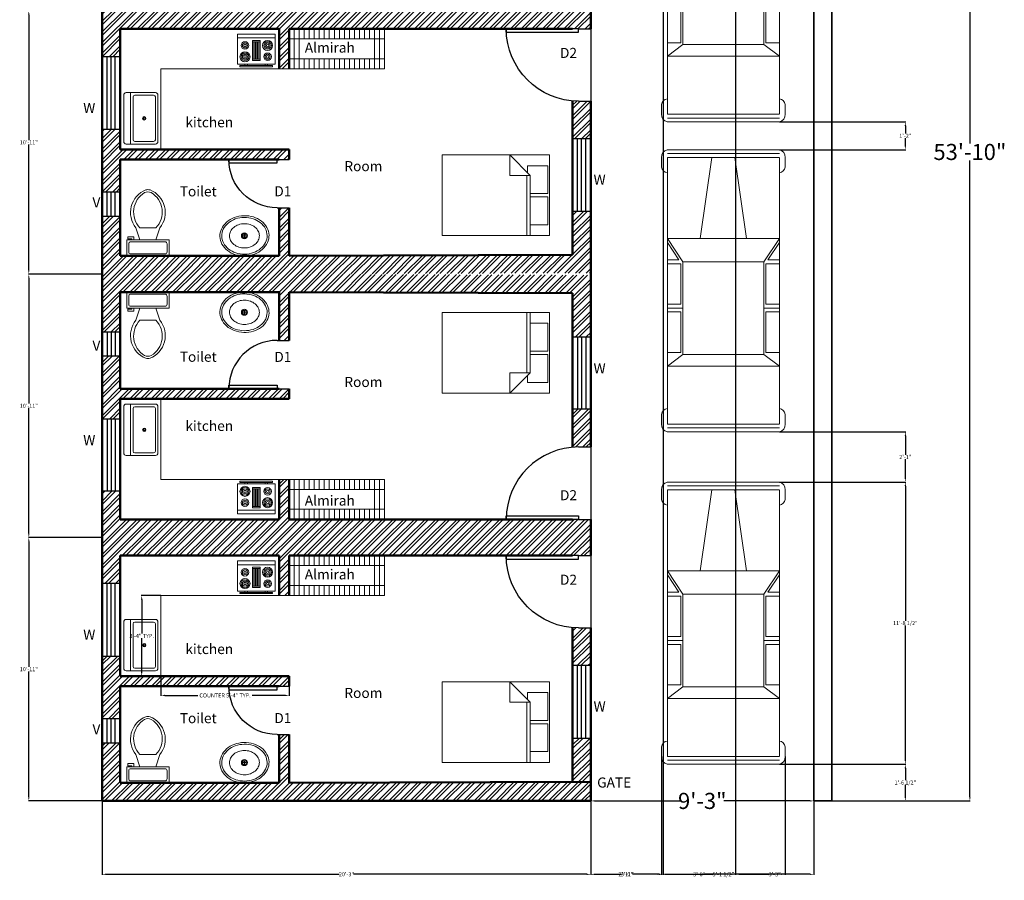
# Model space of a CAD drawing. Units: inches. Extents: x -83 to 408, y 158 to 919.
# Tile 1 of 5: x -82 to 408, y 158 to 586. Entities that reach past the tile are written whole.
import ezdxf

# ---------------------------------------------------------------- set-up
doc = ezdxf.new("R2010")
doc.units = ezdxf.units.IN
doc.header["$MEASUREMENT"] = 0
for name, color, linetype, lineweight in [('A-ANNO-DIMS', 2, 'Continuous', 18), ('A-ANNO-TEXT', 7, 'Continuous', 18), ('A-AREA-IDEN', 7, 'Continuous', 18), ('A-DOOR', 3, 'Continuous', 25), ('A-EQPM', 8, 'Continuous', 18), ('A-FLOR-CASE', 30, 'Continuous', 18), ('A-FLOR-FIXT', 9, 'Continuous', 18), ('A-FURN', 8, 'Continuous', 18), ('A-GLAZ', 4, 'Continuous', 25), ('A-WALL', 7, 'Continuous', 50), ('A-WALL-PATT', 252, 'Continuous', 13), ('C-PKNG-VEHI', 8, 'Continuous', 18), ('L-WALL', 7, 'Continuous', 35)]:
    doc.layers.add(name, color=color, linetype=linetype, lineweight=lineweight)
doc.styles.get("Standard").update_dxf_attribs({"font": 'arial.ttf'})
doc.dimstyles.get("Standard").update_dxf_attribs({"dimtxt": 2, "dimasz": 2, "dimexe": 0.18, "dimexo": 0.0625, "dimgap": 0.09, "dimtad": 0, "dimtih": 1, "dimtoh": 1, "dimdec": 0, "dimzin": 0, "dimdsep": 46, "dimlunit": 3, "dimtxsty": 'Standard', "dimcen": 0.09, "dimadec": 0, "dimazin": 0, "dimtfac": 1, "dimtdec": 0, "dimtofl": 0, "dimtmove": 0, "dimatfit": 3, "dimfxl": 1, "dimtolj": 1, "dimtzin": 0, "dimarcsym": 0})
pattern_1 = [(45, (0, -122.02), (-2.65165, 2.65165), []), (45, (1.7678, -122.02), (-2.65165, 2.65165), [])]

# ---------------------------------------------------------------- blocks, each defined once
blk = doc.blocks.new('Sink - Oval top')
for p, q in [((-1, 0), (1, 0)), ((0, 1), (0, -1))]:
    blk.add_line(p, q)
for points in [[(-12.23, 0.39, 0.117634), (-11.46, -3.36, 0.104469), (-8.88, -6.8, 0.090016), (-5.08, -9.07, 0.08192), (-0.32, -10.02, 0.08192), (4.49, -9.38, 0.090016), (8.42, -7.36, 0.104469), (11.22, -4.09, 0.117634), (12.23, -0.39, 0.117634), (11.46, 3.36, 0.104469), (8.88, 6.8, 0.090016), (5.08, 9.07, 0.08192), (0.32, 10.02, 0.08192), (-4.49, 9.38, 0.090016), (-8.42, 7.36, 0.104469), (-11.22, 4.09, 0.117634)], [(-11.29, 0.16, 0.118622), (-10.52, -3.25, 0.104678), (-8.07, -6.36, 0.089562), (-4.54, -8.37, 0.081185), (-0.13, -9.15, 0.081185), (4.3, -8.49, 0.089562), (7.89, -6.58, 0.104678), (10.42, -3.55, 0.118622), (11.29, -0.16, 0.118622), (10.52, 3.25, 0.104678), (8.07, 6.36, 0.089562), (4.54, 8.37, 0.081185), (0.13, 9.15, 0.081185), (-4.3, 8.49, 0.089562), (-7.89, 6.58, 0.104678), (-10.42, 3.55, 0.118622)], [(-7.42, 0.08, 0.118283), (-6.91, -2.17, 0.104607), (-5.29, -4.21, 0.089718), (-2.97, -5.53, 0.081436), (-0.07, -6.04, 0.081436), (2.84, -5.59, 0.089718), (5.2, -4.33, 0.104607), (6.86, -2.32, 0.118283), (7.42, -0.08, 0.118283), (6.91, 2.17, 0.104607), (5.29, 4.21, 0.089718), (2.97, 5.53, 0.081436), (0.07, 6.04, 0.081436), (-2.84, 5.59, 0.089718), (-5.2, 4.33, 0.104607), (-6.86, 2.32, 0.118283)]]:
    blk.add_lwpolyline(points, format="xyb", close=True)
for radius in [1.5, 1]:
    blk.add_circle((0, 0), radius)
blk = doc.blocks.new('Toilet - top')
for p, q in [((9.5, -6), (9.5, -2)), ((-10, -8.5), (-8, -8.5)), ((-10, -9.5), (-10, -8.5)), ((-7, -9.5), (-10, -9.5)), ((-8, -8.5), (-8, -8)), ((-7, -8), (-7, -9.5)), ((-4, -8), (-6, -14)), ((4, -8), (6, -14)), ((4, -14), (-4, -14))]:
    blk.add_line(p, q)
blk.add_lwpolyline([(10.5, -8), (10.5, 0), (-10.5, 0), (-10.5, -8)], close=True)
for points in [[(-9.5, -2), (-9.5, -6)], [(8.5, -1), (-8.5, -1)], [(-8.5, -7), (8.5, -7)]]:
    blk.add_lwpolyline(points)
for centre, radius, start, end in [((-8.62, -1.88), 0.884, 81.8699, 188.1301), ((8.62, -1.88), 0.884, 351.8699, 98.1301), ((-8.62, -6.12), 0.884, 171.8699, 278.1301), ((8.62, -6.12), 0.884, 261.8699, 8.1301), ((3.52, -21.58), 12.17, 141.4691, 247.9714), ((4.2, -21.82), 11.33, 136.3677, 238.9468), ((-3.52, -21.58), 12.17, 292.0284, 38.5307), ((-4.2, -21.82), 11.33, 301.053, 43.6321), ((0, -27.88), 4, 245.7318, 294.2682), ((0, -29), 4, 254.8605, 285.1395)]:
    blk.add_arc(centre, radius, start, end)
blk = doc.blocks.new('Bed - Queen')
for p, q in [((0, -80.00003), (0, 0)), ((0, 0), (59.99999, 0)), ((59.99999, 0), (59.99999, -80.00003)), ((7.99999, -1.2), (28.79998, -1.2)), ((7.99999, -14.4), (7.99999, -1.2)), ((28.79998, -1.2), (28.79998, -14.4)), ((31.19999, -1.2), (51.99999, -1.2)), ((31.19999, -14.4), (31.19999, -1.2)), ((51.99999, -1.2), (51.99999, -16.4)), ((0, -14.4), (44.8, -14.4)), ((59.99999, -29.6), (44.8, -14.4)), ((44.8, -14.4), (44.8, -29.6)), ((44.8, -16.8), (0, -16.8)), ((51.99999, -16.4), (46.79936, -16.4)), ((44.8, -29.6), (59.99999, -29.6)), ((59.99999, -80.00003), (0, -80.00003))]:
    blk.add_line(p, q)
blk = doc.blocks.new('Sink-single - 30 in top')
blk.add_line((-15, -3.999996), (15, -3.999996))
for points in [[(-13.5, 0), (13.5, 0)], [(-15, -18.499996), (-15, -1.5)], [(-12.5, -5.499996), (12.5, -5.499996)], [(15, -1.5), (15, -18.499996)], [(-13.5, -17.499996), (-13.5, -6.499996)], [(13.5, -6.499996), (13.5, -17.499996)], [(13.5, -19.999996), (-13.5, -19.999996)], [(12.5, -18.499996), (-12.5, -18.499996)]]:
    blk.add_lwpolyline(points)
for radius in [1, 0.5]:
    blk.add_circle((0, -11.999996), radius)
for centre, radius, start, end in [((-13.5, -1.5), 1.5, 90, 180), ((-12.5, -6.499996), 1, 90, 180), ((12.5, -6.499996), 1, 0, 90), ((13.5, -1.5), 1.5, 0, 90), ((-13.5, -18.499996), 1.5, 180, 270), ((-12.5, -17.499996), 1, 180, 270), ((12.5, -17.499996), 1, 270, 0), ((13.5, -18.499996), 1.5, 270, 0)]:
    blk.add_arc(centre, radius, start, end)
blk = doc.blocks.new('Range-Oven - 30 in top')
for p, q in [((0, -3), (30, -3)), ((12, -6), (18, -6)), ((13, -20), (13, -6)), ((14, -6), (14, -20)), ((15, -20), (15, -6)), ((16, -6), (16, -20)), ((17, -20), (17, -6)), ((18, -20), (12, -20)), ((6, -24), (6, -25)), ((8, -25), (8, -24)), ((22, -25), (22, -24)), ((24, -24), (24, -25))]:
    blk.add_line(p, q)
for points in [[(0, -24), (0, 0), (30, 0), (30, -24)], [(12, -21), (12, -5), (18, -5), (18, -21)], [(2, -26), (2, -25), (28, -25), (28, -26)]]:
    blk.add_lwpolyline(points, close=True)
for centre, radius in [((6, -9), 4), ((6, -9), 3), ((6, -9), 2), ((24, -9), 3), ((24, -9), 2), ((6, -18), 3), ((6, -9), 1), ((24, -18), 4), ((24, -18), 3), ((24, -9), 1), ((6, -18), 2), ((6, -18), 1), ((24, -18), 2), ((24, -18), 1)]:
    blk.add_circle(centre, radius)
blk = doc.blocks.new('*U12')
for p, q in [((0, 0), (0, -6)), ((24, 0), (24, -6))]:
    blk.add_line(p, q)
blk.add_lwpolyline([(0, 0), (0, 24), (1.75, 24), (1.75, 0)], close=True)
blk.add_arc((0, 0), 24, 0, 90)
blk = doc.blocks.new('*U13')
for p, q in [((0, 0), (0, -6)), ((36, 0), (36, -6))]:
    blk.add_line(p, q)
blk.add_lwpolyline([(0, 0), (0, 36), (1.75, 36), (1.75, 0)], close=True)
blk.add_arc((0, 0), 36, 0, 90)
blk = doc.blocks.new('*U15')
for p, q in [((5.44, 42.31), (12.12, 42.31)), ((189.69, 42.31), (183.01, 42.31)), ((0.1, -0.41), (0.1, 38.35)), ((2.77, -0.41), (2.77, 38.31)), ((5.44, -0.41), (5.44, 38.24)), ((5.45, 38.31), (16.12, 38.31)), ((16.12, 38.31), (180.34, 38.31)), ((61.52, -0.41), (61.52, 38.31)), ((61.52, 38.31), (77.54, 27.62)), ((64.19, 38.31), (76.2, 30.29)), ((76.2, 30.29), (76.2, 38.31)), ((78.87, 38.31), (78.87, 28.96)), ((106.91, 28.96), (106.91, 38.31)), ((109.58, 27.62), (109.58, 38.31)), ((112.25, 38.31), (112.25, 28.96)), ((140.29, 28.96), (140.29, 38.31)), ((141.62, 27.62), (149.64, 38.31)), ((149.64, -0.41), (149.64, 38.31)), ((189.69, 38.31), (179.01, 38.31)), ((189.69, -0.41), (189.69, 38.24)), ((192.36, -0.41), (192.36, 38.31)), ((195.03, -0.41), (195.03, 38.35)), ((77.54, 27.62), (141.62, 27.62)), ((77.54, -0.41), (77.54, 27.62)), ((78.87, 28.96), (106.91, 28.96)), ((112.25, 28.96), (140.29, 28.96)), ((141.62, -0.41), (141.62, 27.62)), ((5.44, 7.6), (61.52, 15.61)), ((0.1, -0.42), (0.1, -39.18)), ((2.77, -0.41), (2.77, -39.13)), ((5.44, -0.42), (5.44, -39.07)), ((61.52, -0.41), (61.52, -39.13)), ((77.54, -0.41), (77.54, -28.45)), ((141.62, -0.41), (141.62, -28.45)), ((149.64, -0.41), (149.64, -39.13)), ((189.69, -0.42), (189.69, -39.07)), ((192.36, -0.41), (192.36, -39.13)), ((195.03, -0.42), (195.03, -39.18)), ((5.44, -8.42), (61.52, -16.43)), ((61.52, -39.13), (77.54, -28.45)), ((64.19, -39.13), (76.2, -31.12)), ((76.2, -31.12), (76.2, -39.13)), ((77.54, -28.45), (141.62, -28.45)), ((78.87, -39.13), (78.87, -29.79)), ((78.87, -29.79), (106.91, -29.79)), ((106.91, -29.79), (106.91, -39.13)), ((109.58, -28.45), (109.58, -39.13)), ((112.25, -29.79), (140.29, -29.79)), ((112.25, -39.13), (112.25, -29.79)), ((140.29, -29.79), (140.29, -39.13)), ((141.62, -28.45), (149.64, -39.13)), ((5.45, -39.13), (16.12, -39.13)), ((16.12, -39.13), (180.34, -39.13)), ((189.69, -39.13), (179.01, -39.13)), ((5.44, -43.14), (12.12, -43.14)), ((189.69, -43.14), (183.01, -43.14))]:
    blk.add_line(p, q)
for centre, radius, start, end in [((5.06, 37.26), 5.06, 85.64554, 168.0943), ((11.45, 37.64), 4.72, 8.13011, 81.86996), ((183.68, 37.64), 4.72, 98.13004, 171.8699), ((190.07, 37.26), 5.06, 11.90574, 94.35446), ((5.06, -38.09), 5.06, 191.9057, 274.3545), ((11.45, -38.46), 4.72, 278.13, 351.8699), ((183.68, -38.46), 4.72, 188.1301, 261.87), ((190.07, -38.09), 5.06, 265.6455, 348.0943)]:
    blk.add_arc(centre, radius, start, end)
blk = doc.blocks.new('*D16')
at = {"layer": 'A-ANNO-DIMS', "color": 0, "lineweight": -2, "transparency": 16777216}
for p, q in [((202.19, 197.1), (202.19, 196.97)), ((204.19, 197.15), (246.97, 197.15)), ((311.19, 197.15), (268.41, 197.15)), ((313.19, 197.21), (313.19, 197.33))]:
    blk.add_line(p, q, dxfattribs=at)
at = {"layer": 'A-ANNO-DIMS', "color": 0, "transparency": 16777216}
for points in [[(204.19, 197.48), (204.19, 196.82), (202.19, 197.15)], [(311.19, 197.48), (311.19, 196.82), (313.19, 197.15)]]:
    blk.add_solid(points, dxfattribs=at)
at = {"layer": 'Defpoints', "color": 0, "transparency": 16777216}
for p in [(202.19, 197.16), (313.19, 197.15), (313.19, 197.15)]:
    blk.add_point(p, dxfattribs=at)
at = {"layer": 'A-ANNO-DIMS', "color": 0, "transparency": 16777216, "insert": (257.69, 197.15), "char_height": 2, "attachment_point": 5}
blk.add_mtext('\\A1;{\\H4x;9\'-3"}', dxfattribs=at)
blk = doc.blocks.new('*D17')
at = {"layer": 'A-ANNO-DIMS', "color": 0, "lineweight": -2, "transparency": 16777216}
for p, q in [((322.25, 842.67), (390.98, 842.67)), ((390.8, 840.67), (390.8, 524.09)), ((390.8, 199.15), (390.8, 515.73)), ((322.25, 197.15), (390.98, 197.15))]:
    blk.add_line(p, q, dxfattribs=at)
at = {"layer": 'A-ANNO-DIMS', "color": 0, "transparency": 16777216}
for points in [[(390.47, 840.67), (391.14, 840.67), (390.8, 842.67)], [(390.47, 199.15), (391.14, 199.15), (390.8, 197.15)]]:
    blk.add_solid(points, dxfattribs=at)
at = {"layer": 'Defpoints', "color": 0, "transparency": 16777216}
for p in [(322.19, 842.67), (322.19, 197.15), (390.8, 197.15)]:
    blk.add_point(p, dxfattribs=at)
at = {"layer": 'A-ANNO-DIMS', "color": 0, "transparency": 16777216, "insert": (390.8, 519.91), "char_height": 2, "attachment_point": 5}
blk.add_mtext('\\A1;{\\H4x;53\'-10"}', dxfattribs=at)
blk = doc.blocks.new('ALMIRAH-47IN')
for p, q in [((0, 19.88), (47.48, 19.88)), ((0, 19.88), (0, 0)), ((2.48, 19.88), (2.48, 0)), ((4.98, 19.88), (4.98, 0)), ((7.48, 19.88), (7.48, 14.88)), ((9.98, 19.88), (9.98, 14.88)), ((9.98, 19.88), (9.98, 14.88)), ((9.98, 19.88), (9.98, 14.88)), ((12.48, 19.88), (12.48, 14.88)), ((14.98, 19.88), (14.98, 14.88)), ((14.98, 19.88), (14.98, 14.88)), ((17.48, 19.88), (17.48, 14.88)), ((19.98, 19.88), (19.98, 14.88)), ((22.48, 19.88), (22.48, 14.88)), ((22.48, 19.88), (22.48, 14.88)), ((24.98, 19.88), (24.98, 14.88)), ((24.98, 19.88), (24.98, 14.88)), ((27.48, 19.88), (27.48, 14.88)), ((29.98, 19.88), (29.98, 14.88)), ((29.98, 19.88), (29.98, 14.88)), ((29.98, 19.88), (29.98, 14.88)), ((32.48, 19.88), (32.48, 14.88)), ((34.98, 19.88), (34.98, 14.88)), ((37.48, 19.88), (37.48, 14.88)), ((39.98, 19.88), (39.98, 14.88)), ((42.48, 19.88), (42.48, 0)), ((44.98, 19.88), (44.98, 0)), ((47.48, 19.88), (47.48, 0)), ((0, 14.88), (47.48, 14.88)), ((0, 5), (47.48, 5)), ((7.48, 5), (7.48, 0)), ((9.98, 5), (9.98, 0)), ((9.98, 5), (9.98, 0)), ((9.98, 5), (9.98, 0)), ((12.48, 5), (12.48, 0)), ((14.98, 5), (14.98, 0)), ((14.98, 5), (14.98, 0)), ((17.48, 5), (17.48, 0)), ((19.98, 5), (19.98, 0)), ((22.48, 5), (22.48, 0)), ((22.48, 5), (22.48, 0)), ((24.98, 5), (24.98, 0)), ((24.98, 5), (24.98, 0)), ((27.48, 5), (27.48, 0)), ((29.98, 5), (29.98, 0)), ((29.98, 5), (29.98, 0)), ((29.98, 5), (29.98, 0)), ((32.48, 5), (32.48, 0)), ((34.98, 5), (34.98, 0)), ((37.48, 5), (37.48, 0)), ((39.98, 5), (39.98, 0))]:
    blk.add_line(p, q)
blk = doc.blocks.new('WINDOW-36IN')
for p, q in [((2.5, 36), (2.5, 0)), ((4.5, 36), (4.5, 0)), ((6.5, 36), (6.5, 0))]:
    blk.add_line(p, q)
blk.add_lwpolyline([(0, 36), (9, 36), (9, 0), (0, 0)], close=True)
blk = doc.blocks.new('VENT-12IN')
for p, q in [((2.5, 12), (2.5, 0)), ((4.5, 12), (4.5, 0)), ((6.5, 12), (6.5, 0))]:
    blk.add_line(p, q)
blk.add_lwpolyline([(0, 12), (9, 12), (9, 0), (0, 0)], close=True)
blk = doc.blocks.new('COUNTER-L-STUDIO')
for p, q in [((0, 40.12), (0, 40.12)), ((0, 40.12), (0, 0)), ((0, 0), (63.78, 0))]:
    blk.add_line(p, q)
blk = doc.blocks.new('*D39')
at = {"layer": 'A-ANNO-DIMS', "color": 0, "lineweight": -2, "transparency": 16777216}
for p, q in [((-11.59, 259.12), (-11.59, 249.43)), ((52.19, 259.12), (52.19, 249.43)), ((-9.59, 249.61), (6.83, 249.61)), ((50.19, 249.61), (33.77, 249.61))]:
    blk.add_line(p, q, dxfattribs=at)
at = {"layer": 'A-ANNO-DIMS', "color": 0, "transparency": 16777216}
for points in [[(-9.59, 249.95), (-9.59, 249.28), (-11.59, 249.61)], [(50.19, 249.95), (50.19, 249.28), (52.19, 249.61)]]:
    blk.add_solid(points, dxfattribs=at)
at = {"layer": 'Defpoints', "color": 0, "transparency": 16777216}
for p in [(-11.59, 259.18), (52.19, 259.18), (52.19, 249.61)]:
    blk.add_point(p, dxfattribs=at)
at = {"layer": 'A-ANNO-DIMS', "color": 0, "transparency": 16777216, "insert": (20.3, 249.61), "char_height": 2, "attachment_point": 5}
blk.add_mtext('\\A1;COUNTER 5\'-4" TYP.', dxfattribs=at)
blk = doc.blocks.new('*D40')
at = {"layer": 'A-ANNO-DIMS', "color": 0, "lineweight": -2, "transparency": 16777216}
for p, q in [((-11.66, 299.3), (-21.34, 299.3)), ((-21.16, 297.3), (-21.16, 280.35)), ((-21.16, 261.18), (-21.16, 278.13)), ((-11.66, 259.18), (-21.34, 259.18))]:
    blk.add_line(p, q, dxfattribs=at)
at = {"layer": 'A-ANNO-DIMS', "color": 0, "transparency": 16777216}
for points in [[(-21.49, 297.3), (-20.83, 297.3), (-21.16, 299.3)], [(-21.49, 261.18), (-20.83, 261.18), (-21.16, 259.18)]]:
    blk.add_solid(points, dxfattribs=at)
at = {"layer": 'Defpoints', "color": 0, "transparency": 16777216}
for p in [(-11.59, 299.3), (-21.16, 259.18), (-11.59, 259.18)]:
    blk.add_point(p, dxfattribs=at)
at = {"layer": 'A-ANNO-DIMS', "color": 0, "transparency": 16777216, "insert": (-21.16, 279.24), "char_height": 2, "attachment_point": 5}
blk.add_mtext('\\A1;3\'-4" TYP.', dxfattribs=at)
blk = doc.blocks.new('*D41')
at = {"layer": 'A-ANNO-DIMS', "color": 0, "lineweight": -2, "transparency": 16777216}
for p, q in [((-40.81, 197.12), (-40.81, 160.47)), ((202.19, 197.1), (202.19, 160.47)), ((-38.81, 160.65), (77.15, 160.65)), ((200.19, 160.65), (84.23, 160.65))]:
    blk.add_line(p, q, dxfattribs=at)
at = {"layer": 'A-ANNO-DIMS', "color": 0, "transparency": 16777216}
for points in [[(-38.81, 160.98), (-38.81, 160.32), (-40.81, 160.65)], [(200.19, 160.98), (200.19, 160.32), (202.19, 160.65)]]:
    blk.add_solid(points, dxfattribs=at)
at = {"layer": 'Defpoints', "color": 0, "transparency": 16777216}
for p in [(-40.81, 197.18), (202.19, 197.16), (202.19, 160.65)]:
    blk.add_point(p, dxfattribs=at)
at = {"layer": 'A-ANNO-DIMS', "color": 0, "transparency": 16777216, "insert": (80.69, 160.65), "char_height": 2, "attachment_point": 5}
blk.add_mtext('\\A1;20\'-3"', dxfattribs=at)
blk = doc.blocks.new('*D44')
at = {"layer": 'A-ANNO-DIMS', "color": 0, "lineweight": -2, "transparency": 16777216}
for p, q in [((-40.87, 590.18), (-77.49, 590.18)), ((-77.31, 588.18), (-77.31, 525.79)), ((-77.31, 461.18), (-77.31, 523.57)), ((-40.87, 459.18), (-77.49, 459.18))]:
    blk.add_line(p, q, dxfattribs=at)
at = {"layer": 'A-ANNO-DIMS', "color": 0, "transparency": 16777216}
for points in [[(-77.64, 588.18), (-76.98, 588.18), (-77.31, 590.18)], [(-77.64, 461.18), (-76.98, 461.18), (-77.31, 459.18)]]:
    blk.add_solid(points, dxfattribs=at)
at = {"layer": 'Defpoints', "color": 0, "transparency": 16777216}
for p in [(-40.81, 590.18), (-77.31, 459.18), (-40.81, 459.18)]:
    blk.add_point(p, dxfattribs=at)
at = {"layer": 'A-ANNO-DIMS', "color": 0, "transparency": 16777216, "insert": (-77.31, 524.68), "char_height": 2, "attachment_point": 5}
blk.add_mtext('\\A1;10\'-11"', dxfattribs=at)
blk = doc.blocks.new('*D45')
at = {"layer": 'A-ANNO-DIMS', "color": 0, "lineweight": -2, "transparency": 16777216}
for p, q in [((-40.87, 459.18), (-77.49, 459.18)), ((-77.31, 457.18), (-77.31, 394.79)), ((-77.31, 330.18), (-77.31, 392.57)), ((-40.87, 328.18), (-77.49, 328.18))]:
    blk.add_line(p, q, dxfattribs=at)
at = {"layer": 'A-ANNO-DIMS', "color": 0, "transparency": 16777216}
for points in [[(-77.64, 457.18), (-76.98, 457.18), (-77.31, 459.18)], [(-77.64, 330.18), (-76.98, 330.18), (-77.31, 328.18)]]:
    blk.add_solid(points, dxfattribs=at)
at = {"layer": 'Defpoints', "color": 0, "transparency": 16777216}
for p in [(-40.81, 459.18), (-77.31, 328.18), (-40.81, 328.18)]:
    blk.add_point(p, dxfattribs=at)
at = {"layer": 'A-ANNO-DIMS', "color": 0, "transparency": 16777216, "insert": (-77.31, 393.68), "char_height": 2, "attachment_point": 5}
blk.add_mtext('\\A1;10\'-11"', dxfattribs=at)
blk = doc.blocks.new('*D46')
at = {"layer": 'A-ANNO-DIMS', "color": 0, "lineweight": -2, "transparency": 16777216}
for p, q in [((-40.87, 328.18), (-77.49, 328.18)), ((-77.31, 326.18), (-77.31, 263.79)), ((-77.31, 199.18), (-77.31, 261.57)), ((-40.87, 197.18), (-77.49, 197.18))]:
    blk.add_line(p, q, dxfattribs=at)
at = {"layer": 'A-ANNO-DIMS', "color": 0, "transparency": 16777216}
for points in [[(-77.64, 326.18), (-76.98, 326.18), (-77.31, 328.18)], [(-77.64, 199.18), (-76.98, 199.18), (-77.31, 197.18)]]:
    blk.add_solid(points, dxfattribs=at)
at = {"layer": 'Defpoints', "color": 0, "transparency": 16777216}
for p in [(-40.81, 328.18), (-77.31, 197.18), (-40.81, 197.18)]:
    blk.add_point(p, dxfattribs=at)
at = {"layer": 'A-ANNO-DIMS', "color": 0, "transparency": 16777216, "insert": (-77.31, 262.68), "char_height": 2, "attachment_point": 5}
blk.add_mtext('\\A1;10\'-11"', dxfattribs=at)
blk = doc.blocks.new('*D57')
at = {"layer": 'A-ANNO-DIMS', "color": 0, "lineweight": -2, "transparency": 16777216}
for p, q in [((274.19, 685.53), (274.19, 160.47)), ((313.19, 685.53), (313.19, 160.47)), ((276.19, 160.65), (290.94, 160.65)), ((311.19, 160.65), (296.44, 160.65))]:
    blk.add_line(p, q, dxfattribs=at)
at = {"layer": 'A-ANNO-DIMS', "color": 0, "transparency": 16777216}
for points in [[(276.19, 160.98), (276.19, 160.32), (274.19, 160.65)], [(311.19, 160.98), (311.19, 160.32), (313.19, 160.65)]]:
    blk.add_solid(points, dxfattribs=at)
at = {"layer": 'Defpoints', "color": 0, "transparency": 16777216}
for p in [(274.19, 685.59), (313.19, 685.59), (313.19, 160.65)]:
    blk.add_point(p, dxfattribs=at)
at = {"layer": 'A-ANNO-DIMS', "color": 0, "transparency": 16777216, "insert": (293.69, 160.65), "char_height": 2, "attachment_point": 5}
blk.add_mtext('\\A1;3\'-3"', dxfattribs=at)
blk = doc.blocks.new('*D59')
at = {"layer": 'A-ANNO-DIMS', "color": 0, "lineweight": -2, "transparency": 16777216}
for p, q in [((202.19, 769.53), (202.19, 160.47)), ((238.19, 769.53), (238.19, 160.47)), ((204.19, 160.65), (217.44, 160.65)), ((236.19, 160.65), (222.94, 160.65))]:
    blk.add_line(p, q, dxfattribs=at)
at = {"layer": 'A-ANNO-DIMS', "color": 0, "transparency": 16777216}
for points in [[(204.19, 160.98), (204.19, 160.32), (202.19, 160.65)], [(236.19, 160.98), (236.19, 160.32), (238.19, 160.65)]]:
    blk.add_solid(points, dxfattribs=at)
at = {"layer": 'Defpoints', "color": 0, "transparency": 16777216}
for p in [(202.19, 769.59), (238.19, 769.59), (238.19, 160.65)]:
    blk.add_point(p, dxfattribs=at)
at = {"layer": 'A-ANNO-DIMS', "color": 0, "transparency": 16777216, "insert": (220.19, 160.65), "char_height": 2, "attachment_point": 5}
blk.add_mtext('\\A1;3\'-0"', dxfattribs=at)
blk = doc.blocks.new('*D60')
at = {"layer": 'A-ANNO-DIMS', "color": 0, "lineweight": -2, "transparency": 16777216}
for p, q in [((238.19, 805.53), (238.19, 160.47)), ((274.19, 805.53), (274.19, 160.47)), ((240.19, 160.65), (253.44, 160.65)), ((272.19, 160.65), (258.94, 160.65))]:
    blk.add_line(p, q, dxfattribs=at)
at = {"layer": 'A-ANNO-DIMS', "color": 0, "transparency": 16777216}
for points in [[(240.19, 160.98), (240.19, 160.32), (238.19, 160.65)], [(272.19, 160.98), (272.19, 160.32), (274.19, 160.65)]]:
    blk.add_solid(points, dxfattribs=at)
at = {"layer": 'Defpoints', "color": 0, "transparency": 16777216}
for p in [(238.19, 805.59), (274.19, 805.59), (274.19, 160.65)]:
    blk.add_point(p, dxfattribs=at)
at = {"layer": 'A-ANNO-DIMS', "color": 0, "transparency": 16777216, "insert": (256.19, 160.65), "char_height": 2, "attachment_point": 5}
blk.add_mtext('\\A1;3\'-0"', dxfattribs=at)
blk = doc.blocks.new('*D64')
at = {"layer": 'A-ANNO-DIMS', "color": 0, "lineweight": -2, "transparency": 16777216}
for p, q in [((237.43, 219.2), (237.43, 160.47)), ((202.19, 197.1), (202.19, 160.47)), ((204.19, 160.65), (216.27, 160.65)), ((235.43, 160.65), (223.35, 160.65))]:
    blk.add_line(p, q, dxfattribs=at)
at = {"layer": 'A-ANNO-DIMS', "color": 0, "transparency": 16777216}
for points in [[(204.19, 160.98), (204.19, 160.32), (202.19, 160.65)], [(235.43, 160.98), (235.43, 160.32), (237.43, 160.65)]]:
    blk.add_solid(points, dxfattribs=at)
at = {"layer": 'Defpoints', "color": 0, "transparency": 16777216}
for p in [(237.43, 219.26), (202.19, 197.16), (237.43, 160.65)]:
    blk.add_point(p, dxfattribs=at)
at = {"layer": 'A-ANNO-DIMS', "color": 0, "transparency": 16777216, "insert": (219.81, 160.65), "char_height": 2, "attachment_point": 5}
blk.add_mtext('\\A1;2\'-11"', dxfattribs=at)
blk = doc.blocks.new('*D65')
at = {"layer": 'A-ANNO-DIMS', "color": 0, "lineweight": -2, "transparency": 16777216}
for p, q in [((237.43, 219.2), (237.43, 160.47)), ((298.94, 219.2), (298.94, 160.47)), ((239.43, 160.65), (263.11, 160.65)), ((296.94, 160.65), (273.26, 160.65))]:
    blk.add_line(p, q, dxfattribs=at)
at = {"layer": 'A-ANNO-DIMS', "color": 0, "transparency": 16777216}
for points in [[(239.43, 160.98), (239.43, 160.32), (237.43, 160.65)], [(296.94, 160.98), (296.94, 160.32), (298.94, 160.65)]]:
    blk.add_solid(points, dxfattribs=at)
at = {"layer": 'Defpoints', "color": 0, "transparency": 16777216}
for p in [(237.43, 219.26), (298.94, 219.26), (298.94, 160.65)]:
    blk.add_point(p, dxfattribs=at)
at = {"layer": 'A-ANNO-DIMS', "color": 0, "transparency": 16777216, "insert": (268.18, 160.65), "char_height": 2, "attachment_point": 5}
blk.add_mtext('\\A1;5\'-1 1/2"', dxfattribs=at)
blk = doc.blocks.new('*D66')
at = {"layer": 'A-ANNO-DIMS', "color": 0, "lineweight": -2, "transparency": 16777216}
for p, q in [((296.12, 215.42), (358.87, 215.42)), ((358.69, 213.42), (358.69, 207.41)), ((358.69, 199.15), (358.69, 205.16)), ((313.25, 197.15), (358.87, 197.15))]:
    blk.add_line(p, q, dxfattribs=at)
at = {"layer": 'A-ANNO-DIMS', "color": 0, "transparency": 16777216}
for points in [[(358.36, 213.42), (359.02, 213.42), (358.69, 215.42)], [(358.36, 199.15), (359.02, 199.15), (358.69, 197.15)]]:
    blk.add_solid(points, dxfattribs=at)
at = {"layer": 'Defpoints', "color": 0, "transparency": 16777216}
for p in [(296.06, 215.42), (313.19, 197.15), (358.69, 197.15)]:
    blk.add_point(p, dxfattribs=at)
at = {"layer": 'A-ANNO-DIMS', "color": 0, "transparency": 16777216, "insert": (358.69, 206.28), "char_height": 2, "attachment_point": 5}
blk.add_mtext('\\A1;1\'-6 1/2"', dxfattribs=at)
blk = doc.blocks.new('*D67')
at = {"layer": 'A-ANNO-DIMS', "color": 0, "lineweight": -2, "transparency": 16777216}
for p, q in [((296.12, 355.73), (358.87, 355.73)), ((358.69, 353.73), (358.69, 286.7)), ((358.69, 217.42), (358.69, 284.45)), ((296.12, 215.42), (358.87, 215.42))]:
    blk.add_line(p, q, dxfattribs=at)
at = {"layer": 'A-ANNO-DIMS', "color": 0, "transparency": 16777216}
for points in [[(358.36, 353.73), (359.02, 353.73), (358.69, 355.73)], [(358.36, 217.42), (359.02, 217.42), (358.69, 215.42)]]:
    blk.add_solid(points, dxfattribs=at)
at = {"layer": 'Defpoints', "color": 0, "transparency": 16777216}
for p in [(296.06, 355.73), (358.69, 355.73), (296.06, 215.42)]:
    blk.add_point(p, dxfattribs=at)
at = {"layer": 'A-ANNO-DIMS', "color": 0, "transparency": 16777216, "insert": (358.69, 285.58), "char_height": 2, "attachment_point": 5}
blk.add_mtext('\\A1;11\'-8 1/2"', dxfattribs=at)
blk = doc.blocks.new('*D68')
at = {"layer": 'A-ANNO-DIMS', "color": 0, "lineweight": -2, "transparency": 16777216}
for p, q in [((296.12, 380.73), (358.87, 380.73)), ((358.69, 378.73), (358.69, 369.32)), ((358.69, 357.73), (358.69, 367.14)), ((296.12, 355.73), (358.87, 355.73))]:
    blk.add_line(p, q, dxfattribs=at)
at = {"layer": 'A-ANNO-DIMS', "color": 0, "transparency": 16777216}
for points in [[(358.36, 378.73), (359.02, 378.73), (358.69, 380.73)], [(358.36, 357.73), (359.02, 357.73), (358.69, 355.73)]]:
    blk.add_solid(points, dxfattribs=at)
at = {"layer": 'Defpoints', "color": 0, "transparency": 16777216}
for p in [(296.06, 380.73), (358.69, 380.73), (296.06, 355.73)]:
    blk.add_point(p, dxfattribs=at)
at = {"layer": 'A-ANNO-DIMS', "color": 0, "transparency": 16777216, "insert": (358.69, 368.23), "char_height": 2, "attachment_point": 5}
blk.add_mtext('\\A1;2\'-1"', dxfattribs=at)
blk = doc.blocks.new('*D69')
at = {"layer": 'A-ANNO-DIMS', "color": 0, "lineweight": -2, "transparency": 16777216}
for p, q in [((296.12, 534.85), (358.87, 534.85)), ((358.69, 532.85), (358.69, 529.04)), ((358.69, 523.04), (358.69, 526.85)), ((296.12, 521.04), (358.87, 521.04))]:
    blk.add_line(p, q, dxfattribs=at)
at = {"layer": 'A-ANNO-DIMS', "color": 0, "transparency": 16777216}
for points in [[(358.36, 532.85), (359.02, 532.85), (358.69, 534.85)], [(358.36, 523.04), (359.02, 523.04), (358.69, 521.04)]]:
    blk.add_solid(points, dxfattribs=at)
at = {"layer": 'Defpoints', "color": 0, "transparency": 16777216}
for p in [(296.06, 534.85), (358.69, 534.85), (296.06, 521.04)]:
    blk.add_point(p, dxfattribs=at)
at = {"layer": 'A-ANNO-DIMS', "color": 0, "transparency": 16777216, "insert": (358.69, 527.95), "char_height": 2, "attachment_point": 5}
blk.add_mtext('\\A1;1\'-2"', dxfattribs=at)

msp = doc.modelspace()

# ---------------------------------------------------------------- hatches: boundary and pattern name
at = {"layer": 'A-WALL-PATT'}
h = msp.add_hatch(dxfattribs=at)
h.set_pattern_fill('ANSI32', color=256, scale=10)
h.set_pattern_definition(pattern_1)
h.paths.add_polyline_path([(202.19, 459.71), (52.21, 459.18), (-40.81, 459.18), (-40.81, 487.99), (-31.81, 487.99), (-31.81, 468.18), (47.19, 468.18), (47.19, 492.18), (52.19, 492.18), (52.19, 468.18), (193.19, 468.68), (193.19, 490.43), (202.19, 490.43)])
h.paths.add_polyline_path([(202.19, 526.43), (193.19, 526.43), (193.19, 545.31, 0.020861), (196.19, 545.18), (202.19, 545.18)])
h.paths.add_polyline_path([(202.19, 581.18), (196.19, 581.18), (160.19, 581.18), (52.19, 581.18), (52.19, 561.3), (47.19, 561.3), (47.19, 581.18), (-31.81, 581.18), (-31.81, 567.22), (-40.81, 567.22), (-40.81, 590.18), (202.19, 590.18)])
h.paths.add_polyline_path([(52.19, 516.18), (46.19, 516.18), (22.19, 516.18), (-31.81, 516.18), (-31.81, 499.99), (-40.81, 499.99), (-40.81, 531.22), (-31.81, 531.22), (-31.81, 521.18), (52.19, 521.18)])
h = msp.add_hatch(dxfattribs=at)
h.set_pattern_fill('ANSI32', color=256, scale=10)
h.set_pattern_definition(pattern_1)
h.paths.add_polyline_path([(202.19, 458.65), (52.21, 459.18), (-40.81, 459.18), (-40.81, 430.37), (-31.81, 430.37), (-31.81, 450.18), (47.19, 450.18), (47.19, 426.18), (52.19, 426.18), (52.19, 450.18), (193.19, 449.68), (193.19, 427.93), (202.19, 427.93)])
h.paths.add_polyline_path([(202.19, 391.93), (193.19, 391.93), (193.19, 373.05, -0.020861), (196.19, 373.18), (202.19, 373.18)])
h.paths.add_polyline_path([(202.19, 337.18), (196.19, 337.18), (160.19, 337.18), (52.19, 337.18), (52.19, 357.06), (47.19, 357.06), (47.19, 337.18), (-31.81, 337.18), (-31.81, 351.14), (-40.81, 351.14), (-40.81, 328.18), (202.19, 328.18)])
h.paths.add_polyline_path([(52.19, 402.18), (46.19, 402.18), (22.19, 402.18), (-31.81, 402.18), (-31.81, 418.37), (-40.81, 418.37), (-40.81, 387.14), (-31.81, 387.14), (-31.81, 397.18), (52.19, 397.18)])
h = msp.add_hatch(dxfattribs=at)
h.set_pattern_fill('ANSI32', color=256, scale=10)
h.set_pattern_definition(pattern_1)
h.paths.add_polyline_path([(202.19, 197.71), (52.21, 197.18), (-40.81, 197.18), (-40.81, 225.99), (-31.81, 225.99), (-31.81, 206.18), (47.19, 206.18), (47.19, 230.18), (52.19, 230.18), (52.19, 206.18), (193.19, 206.68), (193.19, 228.43), (202.19, 228.43)])
h.paths.add_polyline_path([(202.19, 264.43), (193.19, 264.43), (193.19, 283.31, 0.020861), (196.19, 283.18), (202.19, 283.18)])
h.paths.add_polyline_path([(202.19, 319.18), (196.19, 319.18), (160.19, 319.18), (52.19, 319.18), (52.19, 299.3), (47.19, 299.3), (47.19, 319.18), (-31.81, 319.18), (-31.81, 305.22), (-40.81, 305.22), (-40.81, 328.18), (202.19, 328.18)])
h.paths.add_polyline_path([(52.19, 254.18), (46.19, 254.18), (22.19, 254.18), (-31.81, 254.18), (-31.81, 237.99), (-40.81, 237.99), (-40.81, 269.22), (-31.81, 269.22), (-31.81, 259.18), (52.19, 259.18)])

# ---------------------------------------------------------------- linework, layer by layer
at = {"layer": 'A-WALL'}
for p, q in [((-40.81, 590.18), (-40.81, 459.18)), ((202.19, 590.18), (202.19, 581.18)), ((-40.81, 450.2), (-40.81, 581.2)), ((47.19, 581.18), (-31.81, 581.18)), ((-31.81, 581.18), (-31.81, 521.18)), ((47.19, 561.3), (47.19, 581.18)), ((52.19, 561.3), (52.19, 581.18)), ((52.19, 581.18), (193.19, 581.18)), ((193.19, 545.31), (193.19, 468.68)), ((202.19, 545.18), (202.19, 459.71)), ((47.19, 521.18), (-31.81, 521.18)), ((-31.81, 521.18), (52.19, 521.18)), ((52.19, 516.18), (52.19, 521.18)), ((52.19, 516.18), (52.19, 521.18)), ((47.19, 516.18), (-31.81, 516.18)), ((-31.81, 516.18), (-31.81, 468.18)), ((-31.81, 516.18), (47.19, 516.18)), ((47.19, 468.18), (47.19, 492.18)), ((52.19, 468.18), (52.19, 492.18)), ((52.19, 468.18), (52.19, 492.18)), ((-40.81, 468.16), (-40.81, 337.16)), ((-31.81, 468.18), (47.19, 468.18)), ((193.19, 468.68), (52.19, 468.18)), ((202.19, 468.16), (202.19, 459.16)), ((-40.81, 328.18), (-40.81, 459.18)), ((202.19, 450.2), (202.19, 459.2)), ((202.19, 373.18), (202.19, 458.65)), ((-31.81, 450.18), (47.19, 450.18)), ((-31.81, 402.18), (-31.81, 450.18)), ((47.19, 450.18), (47.19, 426.18)), ((52.19, 450.18), (52.19, 426.18)), ((193.19, 449.68), (52.19, 450.18)), ((52.19, 450.18), (52.19, 426.18)), ((193.19, 373.05), (193.19, 449.68)), ((47.19, 402.18), (-31.81, 402.18)), ((-31.81, 402.18), (47.19, 402.18)), ((52.19, 402.18), (52.19, 397.18)), ((52.19, 402.18), (52.19, 397.18)), ((47.19, 397.18), (-31.81, 397.18)), ((-31.81, 397.18), (52.19, 397.18)), ((-31.81, 337.18), (-31.81, 397.18)), ((47.19, 357.06), (47.19, 337.18)), ((52.19, 357.06), (52.19, 337.18)), ((47.19, 337.18), (-31.81, 337.18)), ((52.19, 337.18), (193.19, 337.18)), ((202.19, 328.18), (202.19, 337.18)), ((-40.81, 328.18), (-40.81, 197.18)), ((202.19, 328.18), (202.19, 319.18)), ((-40.81, 197.18), (-40.81, 319.2)), ((47.19, 319.18), (-31.81, 319.18)), ((-31.81, 319.18), (-31.81, 259.18)), ((47.19, 299.3), (47.19, 319.18)), ((52.19, 299.3), (52.19, 319.18)), ((52.19, 319.18), (193.19, 319.18)), ((193.19, 283.31), (193.19, 206.68)), ((202.19, 283.18), (202.19, 197.71)), ((47.19, 259.18), (-31.81, 259.18)), ((-31.81, 259.18), (52.19, 259.18)), ((52.19, 254.18), (52.19, 259.18)), ((52.19, 254.18), (52.19, 259.18)), ((47.19, 254.18), (-31.81, 254.18)), ((-31.81, 254.18), (-31.81, 206.18)), ((-31.81, 254.18), (47.19, 254.18)), ((47.19, 206.18), (47.19, 230.18)), ((52.19, 206.18), (52.19, 230.18)), ((52.19, 206.18), (52.19, 230.18)), ((-31.81, 206.18), (47.19, 206.18)), ((202.19, 206.71), (52.19, 206.18)), ((202.19, 206.16), (202.19, 197.16)), ((202.19, 197.16), (-40.81, 197.18))]:
    msp.add_line(p, q, dxfattribs=at)
at = {"layer": 'L-WALL'}
for p, q in [((322.19, 842.67), (322.19, 197.15)), ((313.19, 833.67), (313.19, 197.15)), ((322.19, 197.15), (313.19, 197.15))]:
    msp.add_line(p, q, dxfattribs=at)

# ---------------------------------------------------------------- block references
at = {"layer": 'A-DOOR', "xscale": -1}
for name, p, rotation in [('*U13', (196.19, 581.18), 90), ('*U12', (46.19, 516.18), 90), ('*U13', (196.19, 319.18), 89.99999999999991), ('*U12', (46.19, 254.18), 89.99999999999991)]:
    msp.add_blockref(name, p, dxfattribs=dict(at, rotation=rotation))
at = {"layer": 'A-DOOR', "rotation": 90.00000000000006}
for name, p in [('*U12', (46.19, 402.18)), ('*U13', (196.19, 337.18))]:
    msp.add_blockref(name, p, dxfattribs=at)
at = {"layer": 'A-EQPM', "xscale": -0.6253442555691314, "yscale": 0.6253442555691314, "zscale": 0.6253442555691314}
for p in [(45.23, 578.5), (45.23, 316.5)]:
    msp.add_blockref('Range-Oven - 30 in top', p, dxfattribs=at)
at = {"layer": 'A-EQPM', "xscale": 0.6253442555691314, "yscale": 0.6253442555691314, "zscale": 0.6253442555691314, "rotation": 180}
msp.add_blockref('Range-Oven - 30 in top', (45.23, 339.86), dxfattribs=at)
at = {"layer": 'A-FLOR-CASE', "extrusion": (0, 0, -1), "zscale": -1, "rotation": 180}
for name, p in [('ALMIRAH-47IN', (-52.19, 581.18)), ('COUNTER-L-STUDIO', (11.59, 561.3)), ('ALMIRAH-47IN', (-52.19, 319.18)), ('COUNTER-L-STUDIO', (11.59, 299.3))]:
    msp.add_blockref(name, p, dxfattribs=at)
at = {"layer": 'A-FLOR-CASE'}
for name, p in [('COUNTER-L-STUDIO', (-11.59, 357.06)), ('ALMIRAH-47IN', (52.19, 337.18))]:
    msp.add_blockref(name, p, dxfattribs=at)
at = {"layer": 'A-FLOR-FIXT', "yscale": 0.8513407291768876, "zscale": 0.8513407291768876}
for p, xscale, rotation in [((-30.11, 536.63), -0.8513407291768876, 90), ((-30.11, 381.73), 0.8513407291768876, 90.00000000000006), ((-30.11, 274.63), -0.8513407291768876, 89.99999999999991)]:
    msp.add_blockref('Sink-single - 30 in top', p, dxfattribs=dict(at, xscale=xscale, rotation=rotation))
at = {"layer": 'A-FLOR-FIXT', "xscale": -1, "rotation": 180}
for name, p in [('Toilet - top', (-18.06, 468.18)), ('Sink - Oval top', (29.95, 478.2)), ('Toilet - top', (-18.06, 206.18)), ('Sink - Oval top', (29.95, 216.2))]:
    msp.add_blockref(name, p, dxfattribs=at)
at = {"layer": 'A-FLOR-FIXT'}
for name, p in [('Toilet - top', (-18.06, 450.18)), ('Sink - Oval top', (29.95, 440.16))]:
    msp.add_blockref(name, p, dxfattribs=at)
at = {"layer": 'A-FURN', "yscale": 0.667678018977486, "zscale": 0.667678018977486}
for p, xscale, rotation in [((181.69, 478.34), -0.667678018977486, 270), ((181.69, 440.02), 0.667678018977486, 270.0000000000001), ((181.69, 216.34), -0.667678018977486, 269.9999999999999)]:
    msp.add_blockref('Bed - Queen', p, dxfattribs=dict(at, xscale=xscale, rotation=rotation))
at = {"layer": 'A-GLAZ', "extrusion": (0, 0, -1), "zscale": -1, "rotation": 180}
for name, p in [('WINDOW-36IN', (40.81, 567.22)), ('WINDOW-36IN', (-193.19, 526.43)), ('VENT-12IN', (40.81, 499.99)), ('WINDOW-36IN', (40.81, 305.22)), ('WINDOW-36IN', (-193.19, 264.43)), ('VENT-12IN', (40.81, 237.99))]:
    msp.add_blockref(name, p, dxfattribs=at)
at = {"layer": 'A-GLAZ'}
for name, p in [('VENT-12IN', (-40.81, 418.37)), ('WINDOW-36IN', (193.19, 391.93)), ('WINDOW-36IN', (-40.81, 351.14))]:
    msp.add_blockref(name, p, dxfattribs=at)
at = {"layer": 'C-PKNG-VEHI', "xscale": 0.7198545955529133, "yscale": 0.7198545955529133, "zscale": 0.7198545955529133, "rotation": 270}
for p in [(268.48, 675.24), (268.48, 521.12), (268.48, 355.81)]:
    msp.add_blockref('*U15', p, dxfattribs=at)

# ---------------------------------------------------------------- texts
at = {"layer": 'A-ANNO-TEXT', "char_height": 5}
for s, width, insert, attachment_point in [('Almirah', 24.1185, (59.97, 569.32), 7), ('D2', 13.3697, (186.91, 566.67), 7), ('W', 4.9358, (-50.22, 539.3), 7), ('W', 4.9358, (203.62, 503.62), 7), ('D1', 13.3697, (44.82, 497.86), 7), ('V', 4.2263, (-45.64, 492.31), 7), ('V', 4.2263, (-45.64, 426.05), 1), ('D1', 13.3697, (44.82, 420.5), 1), ('W', 4.9358, (203.62, 414.74), 1), ('W', 4.9358, (-50.22, 379.06), 1), ('Almirah', 24.1185, (59.97, 349.04), 1), ('D2', 13.3697, (186.91, 351.69), 1), ('Almirah', 24.1185, (59.97, 307.32), 7), ('D2', 13.3697, (186.91, 304.67), 7), ('W', 4.9358, (-50.22, 277.3), 7), ('W', 4.9358, (203.62, 241.62), 7), ('D1', 13.3697, (44.82, 235.86), 7), ('V', 4.2263, (-45.64, 230.31), 7)]:
    msp.add_mtext_dynamic_manual_height_columns(s, width=width, gutter_width=1, heights=[0], dxfattribs=dict(at, insert=insert, attachment_point=attachment_point))
at = {"layer": 'A-ANNO-TEXT', "insert": (205.4, 208.8), "char_height": 5, "attachment_point": 1}
msp.add_mtext('GATE', dxfattribs=at)
at = {"layer": 'A-AREA-IDEN', "char_height": 5}
for s, width, heights, insert, attachment_point in [('kitchen', 18.1432, [0], (0.57, 532.19), 7), ('Room', 29.7735, [0], (79.66, 510.35), 7), ('Toilet', 21.3997, [0.203], (-2.22, 497.81), 7), ('Toilet', 21.3997, [0.203], (-2.22, 420.55), 1), ('Room', 29.7735, [0], (79.66, 408.01), 1), ('kitchen', 18.1432, [0], (0.57, 386.17), 1), ('kitchen', 18.1432, [0], (0.57, 270.19), 7), ('Room', 29.7735, [0], (79.66, 248.35), 7), ('Toilet', 21.3997, [0.203], (-2.22, 235.81), 7)]:
    msp.add_mtext_dynamic_manual_height_columns(s, width=width, gutter_width=1, heights=heights, dxfattribs=dict(at, insert=insert, attachment_point=attachment_point))

# ---------------------------------------------------------------- dimensions: what is measured, and where the dimension line sits
at = {"layer": 'A-ANNO-DIMS'}
for base, p1, p2, angle, text, override, picture, middle in [((390.8, 197.15), (322.19, 842.67), (322.19, 197.15), 90, '{\\H4x;<>}', {"dimclrd": 0, "dimclre": 0, "dimclrt": 0}, '*D17', (390.8, 519.91)), ((-21.16, 259.18), (-11.59, 299.3), (-11.59, 259.18), 270, '<> TYP.', {"dimdec": 1, "dimlfac": 1, "dimrnd": 0, "dimzin": 1, "dimdsep": 46, "dimlunit": 4, "dimfrac": 2}, '*D40', (-21.16, 279.24))]:
    dim = msp.add_linear_dim(base=base, p1=p1, p2=p2, angle=angle, text=text, dimstyle='Standard', override=override, dxfattribs=at)
    dim.commit()
    dim.dimension.update_dxf_attribs({"geometry": picture, "text_midpoint": middle})
for base, p1, p2, picture, middle in [((274.19, 160.65), (238.19, 805.59), (274.19, 805.59), '*D60', (256.19, 160.65)), ((238.19, 160.65), (202.19, 769.59), (238.19, 769.59), '*D59', (220.19, 160.65)), ((313.19, 160.65), (274.19, 685.59), (313.19, 685.59), '*D57', (293.69, 160.65)), ((237.43, 160.65), (202.19, 197.16), (237.43, 219.26), '*D64', (219.81, 160.65)), ((298.94, 160.65), (237.43, 219.26), (298.94, 219.26), '*D65', (268.18, 160.65)), ((202.19, 160.65), (-40.81, 197.18), (202.19, 197.16), '*D41', (80.69, 160.65))]:
    dim = msp.add_linear_dim(base=base, p1=p1, p2=p2, dimstyle='Standard', override={"dimdec": 1, "dimlfac": 1, "dimrnd": 0, "dimzin": 1, "dimdsep": 46, "dimlunit": 4, "dimfrac": 2}, dxfattribs=at)
    dim.commit()
    dim.dimension.update_dxf_attribs({"geometry": picture, "text_midpoint": middle})
for base, p1, p2, picture, middle in [((-77.31, 459.18), (-40.81, 590.18), (-40.81, 459.18), '*D44', (-77.31, 524.68)), ((358.69, 534.85), (296.06, 521.04), (296.06, 534.85), '*D69', (358.69, 527.95)), ((-77.31, 328.18), (-40.81, 459.18), (-40.81, 328.18), '*D45', (-77.31, 393.68)), ((358.69, 380.73), (296.06, 355.73), (296.06, 380.73), '*D68', (358.69, 368.23)), ((358.69, 355.73), (296.06, 215.42), (296.06, 355.73), '*D67', (358.69, 285.58)), ((-77.31, 197.18), (-40.81, 328.18), (-40.81, 197.18), '*D46', (-77.31, 262.68)), ((358.69, 197.15), (296.06, 215.42), (313.19, 197.15), '*D66', (358.69, 206.28))]:
    dim = msp.add_linear_dim(base=base, p1=p1, p2=p2, angle=90, dimstyle='Standard', override={"dimdec": 1, "dimlfac": 1, "dimrnd": 0, "dimzin": 1, "dimdsep": 46, "dimlunit": 4, "dimfrac": 2}, dxfattribs=at)
    dim.commit()
    dim.dimension.update_dxf_attribs({"geometry": picture, "text_midpoint": middle})
for base, p1, p2, text, override, picture, middle in [((52.19, 249.61), (-11.59, 259.18), (52.19, 259.18), 'COUNTER <> TYP.', {"dimdec": 1, "dimlfac": 1, "dimrnd": 0, "dimzin": 1, "dimdsep": 46, "dimlunit": 4, "dimfrac": 2}, '*D39', (20.3, 249.61)), ((313.19, 197.15), (202.19, 197.16), (313.19, 197.15), '{\\H4x;<>}', {"dimclrd": 0, "dimclre": 0, "dimclrt": 0}, '*D16', (257.69, 197.15))]:
    dim = msp.add_linear_dim(base=base, p1=p1, p2=p2, text=text, dimstyle='Standard', override=override, dxfattribs=at)
    dim.commit()
    dim.dimension.update_dxf_attribs({"geometry": picture, "text_midpoint": middle})

doc.saveas('drawing.dxf')
